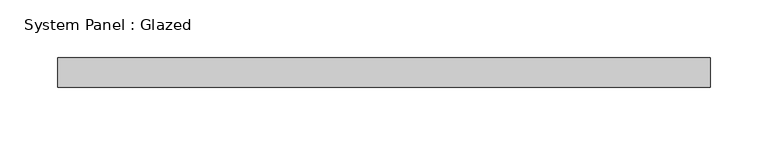
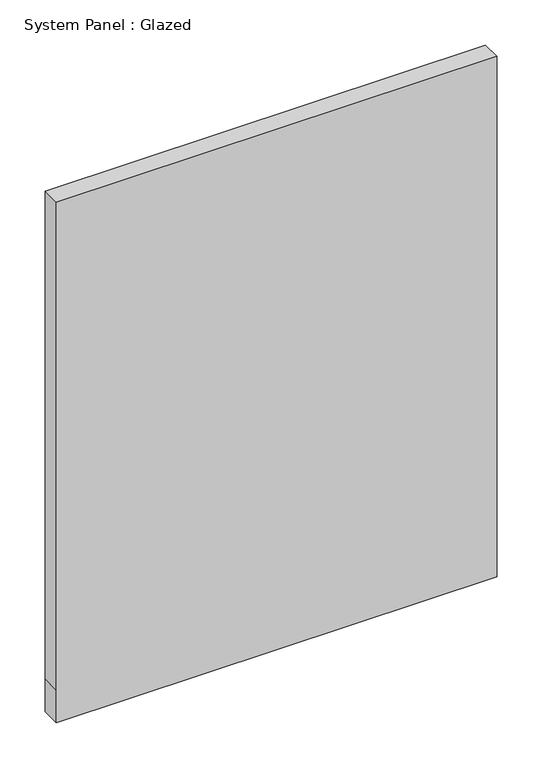
"""IFC4 building model written with IfcOpenShell, lengths in millimetres: plate geometry, System Panel : Glazed."""

from ifc_helpers import new_model, si_unit, frame, origin, place, context, project, spatial, polyline, outline, extrude, source, transform, mapped, element, save


def system_panel_glazed_474a16cc(model_context):
    return source(origin(), model_context, "Body", "SweptSolid", [
        extrude(outline(polyline([(0.0, -282.575), (0.0, 282.575), (44.45, 282.575), (705.6801773, 282.575), (705.6801773, -282.575), (44.45, -282.575), (0.0, -282.575)])), frame((0.0, 19.05, 0.0), z_axis=(0.0, 1.0, 0.0), x_axis=(0.0, 0.0, 1.0)), (0.0, 0.0, 1.0), 25.4),
    ])


if __name__ == "__main__":
    model = new_model("IFC4")
    model_context = context("Model", 3, world=origin())
    ifc_project = project(units=[si_unit("LENGTHUNIT", "METRE", prefix="MILLI")], contexts=[model_context])
    site = spatial("IfcSite", under=ifc_project)
    building = spatial("IfcBuilding", under=site)
    placement = place(None, origin())
    system_panel_glazed_shape = system_panel_glazed_474a16cc(model_context)
    element("IfcPlate", 1, ObjectType="System Panel : Glazed", at=placement, inside=building, context=model_context, shape_type="MappedRepresentation", body=[
        mapped(system_panel_glazed_shape, transform((0.0, 0.0, 0.0), x_axis=(1.0, 0.0, 0.0), y_axis=(0.0, 1.0, 0.0), z_axis=(0.0, 0.0, 1.0))),
    ])
    save(model, "model.ifc")

# Revit data of these elements
# Type "System Panel : Glazed"
#   Construction Type Id = "GSP4R"
#   Analytic Construction = "1/8 in Pilkington single glazing"
#   Visual Light Transmittance = 0.9
#   Solar Heat Gain Coefficient = 0.86
#   Heat Transfer Coefficient (U) = 1.18115 BTU/(h·ft²·°F)
#   Define Thermal Properties by = 1
# Element 1 (IfcPlate, "System Panel : Glazed")
#   Materials on its faces: "Glass"
# Materials
#   "Glass": class "Glass", colour RGB 0 128 192, transparency 0.75, Description = "Soda Lime Glass", Cost = 0
